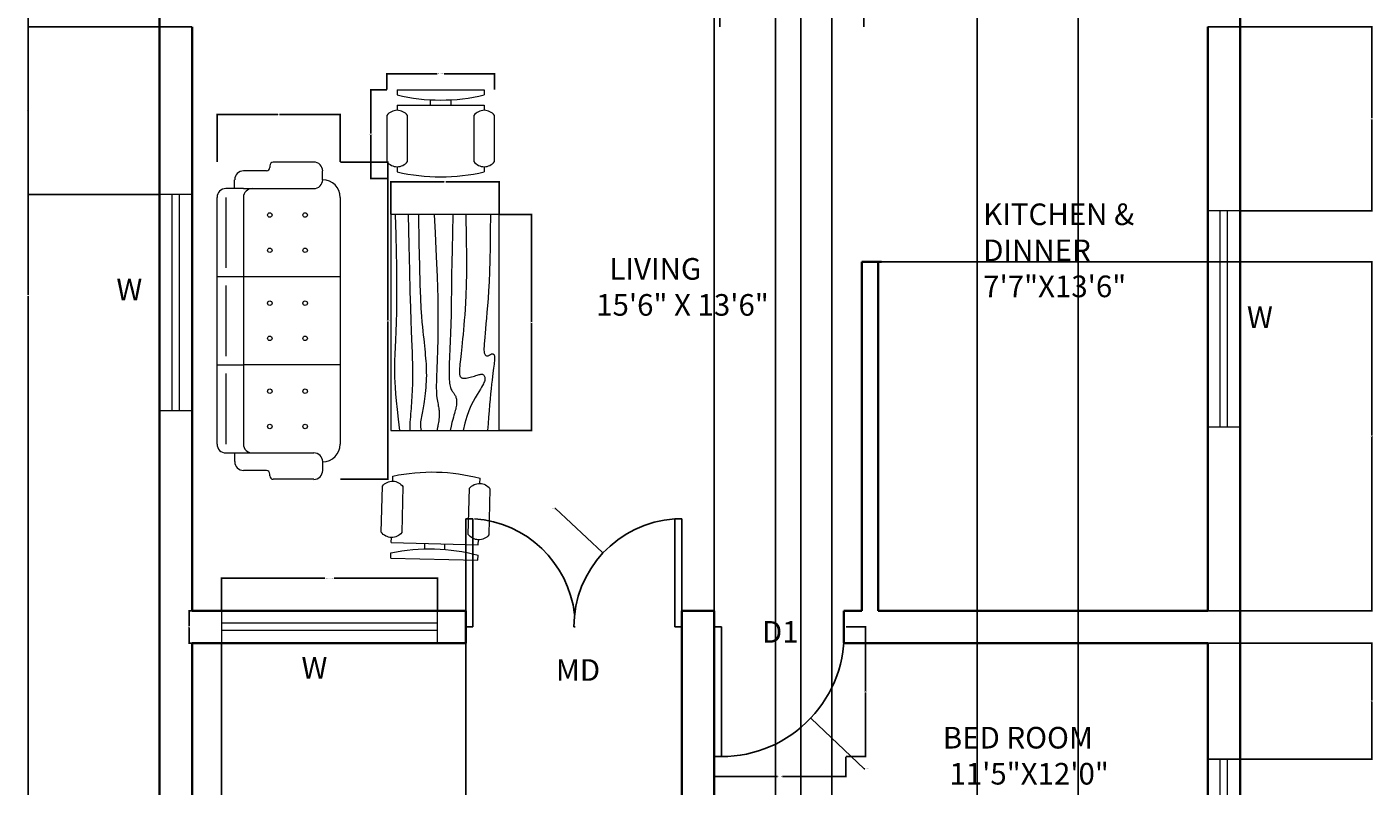
# Model space of a CAD drawing. Units: inches. Extents: x 2523 to 5630, y 2079 to 4208.
# Tile 2 of 3: x 2523 to 2897, y 2309 to 2520. Entities that reach past the tile are written whole.
import ezdxf

# ---------------------------------------------------------------- set-up
doc = ezdxf.new("R2010")
doc.units = ezdxf.units.IN
for name, color, linetype, lineweight in [('A-ANNO-DIMS', 2, 'Continuous', 18), ('A-ANNO-TEXT', 7, 'Continuous', 18), ('A-AREA-IDEN', 7, 'Continuous', 25), ('A-DOOR', 3, 'Continuous', 25), ('A-FURN', 8, 'Continuous', 18), ('A-GLAZ', 4, 'Continuous', 18), ('A-WALL', 7, 'Continuous', 35)]:
    doc.layers.add(name, color=color, linetype=linetype, lineweight=lineweight)
doc.styles.get("Standard").update_dxf_attribs({"font": 'arial.ttf'})
doc.dimstyles.get("Standard").update_dxf_attribs({"dimtxt": 0.18, "dimasz": 0.18, "dimexe": 0.18, "dimexo": 0.0625, "dimgap": 0.09, "dimtad": 0, "dimtih": 1, "dimtoh": 1, "dimdec": 4, "dimzin": 0, "dimdsep": 46, "dimtxsty": 'Standard', "dimcen": 0.09, "dimadec": 0, "dimazin": 0, "dimtfac": 1, "dimtdec": 4, "dimtofl": 0, "dimtmove": 0, "dimatfit": 3, "dimfxl": 1, "dimtolj": 1, "dimtzin": 0, "dimarcsym": 0})

# ---------------------------------------------------------------- blocks, each defined once
blk = doc.blocks.new('A$C1BE21B70')
for p, q in [((0.269, 0.942), (2.154, 0.942)), ((0.875, 0.942), (0.875, 0.875)), ((1.548, 0), (1.548, 0.942)), ((0.202, 0.875), (0.202, 0.74)), ((0.808, 0.875), (0.269, 0.875)), ((0.875, 0.875), (0.875, 0.74)), ((1.481, 0.875), (0.942, 0.875)), ((2.154, 0.875), (1.616, 0.875)), ((2.221, 0.74), (2.221, 0.875)), ((0.067, 0.565), (0.067, 0.74)), ((0.202, 0.808), (0.135, 0.808)), ((0.202, 0.74), (0.202, 0.202)), ((2.154, 0.74), (0.269, 0.74)), ((0.875, 0), (0.875, 0.74)), ((2.221, 0.808), (2.289, 0.808)), ((2.221, 0.74), (2.221, 0.202)), ((2.356, 0.565), (2.356, 0.74)), ((0.027, 0.539), (0.04, 0.539)), ((2.396, 0.539), (2.383, 0.539)), ((0, 0.202), (0, 0.512)), ((2.423, 0.202), (2.423, 0.512)), ((0.135, 0.135), (0.067, 0.135)), ((2.289, 0.135), (2.356, 0.135)), ((2.154, 0), (0.269, 0))]:
    blk.add_line(p, q)
for centre in [(0.404, 0.539), (0.673, 0.539), (1.077, 0.539), (1.346, 0.539), (1.75, 0.539), (2.019, 0.539), (0.404, 0.269), (0.673, 0.269), (1.077, 0.269), (1.346, 0.269), (1.75, 0.269), (2.019, 0.269)]:
    blk.add_circle(centre, 0.0171)
for centre, radius, start, end in [((0.269, 0.875), 0.0673, 90, 180), ((2.154, 0.875), 0.0673, 0, 90), ((0.135, 0.74), 0.0673, 90, 180), ((0.269, 0.673), 0.0673, 90, 180), ((2.154, 0.673), 0.0673, 0, 90), ((2.289, 0.74), 0.0673, 0, 90), ((0.027, 0.512), 0.0269, 90, 180), ((0.04, 0.565), 0.0269, 270, 0), ((2.383, 0.565), 0.0269, 180, 270), ((2.396, 0.512), 0.0269, 0, 90), ((0.067, 0.202), 0.0673, 180, 270), ((0.135, 0.202), 0.0673, 270, 0), ((0.269, 0.135), 0.135, 180, 270), ((2.154, 0.135), 0.135, 270, 0), ((2.289, 0.202), 0.0673, 180, 270), ((2.356, 0.202), 0.0673, 270, 0)]:
    blk.add_arc(centre, radius, start, end)
blk = doc.blocks.new('Table - Rectangular Woodgrain 60 x 30 in.')
for p, q in [((0, 0), (0, -30)), ((60, 0), (0, 0)), ((60, -30), (60, 0)), ((0, -30), (60, -30))]:
    blk.add_line(p, q)
for points in [[(0, -2.4), (4.8155, -2.418), (9.0302, -2.4688), (12.709, -2.5477), (15.9167, -2.65), (18.7181, -2.7711), (21.1781, -2.9063), (23.3616, -3.0508), (25.3333, -3.2), (27.1477, -3.3495), (28.8172, -3.4958), (30.3437, -3.636), (31.7291, -3.7667), (32.9756, -3.8849), (34.0849, -3.9875), (35.059, -4.0714), (35.9, -4.1334), (36.6114, -4.1711), (37.2041, -4.1854), (37.6906, -4.1779), (38.0833, -4.15), (38.3948, -4.1034), (38.6375, -4.0396), (38.8239, -3.9602), (38.9666, -3.8667), (39.0764, -3.7608), (39.1573, -3.6448), (39.2116, -3.521), (39.2416, -3.3917), (39.2498, -3.2593), (39.2385, -3.1261), (39.21, -2.9944), (39.1666, -2.8667), (39.111, -2.7447), (39.0468, -2.6281), (38.978, -2.5163), (38.9083, -2.4083), (38.8418, -2.3035), (38.7823, -2.201), (38.7337, -2.1001), (38.7, -2), (38.6844, -1.9003), (38.6875, -1.8021), (38.7094, -1.707), (38.75, -1.6167), (38.8094, -1.5326), (38.8875, -1.4563), (38.9844, -1.3893), (39.1, -1.3333), (39.2351, -1.2896), (39.3937, -1.2583), (39.5804, -1.2396), (39.8, -1.2333), (40.057, -1.2396), (40.3562, -1.2583), (40.7023, -1.2896), (41.1, -1.3333), (41.5547, -1.3895), (42.0755, -1.4573), (42.6721, -1.5361), (43.3542, -1.625), (44.1316, -1.7233), (45.014, -1.8302), (46.0114, -1.9449), (47.1333, -2.0667), (48.3862, -2.1947), (49.7625, -2.3281), (51.2513, -2.4663), (52.8416, -2.6083), (54.5226, -2.7535), (56.2833, -2.9011), (58.1127, -3.0501), (60, -3.2)], [(0, -9.2), (6.5759, -9.0858), (11.9385, -9.0365), (16.2527, -9.0418), (19.6833, -9.0917), (22.3952, -9.1759), (24.5531, -9.2844), (26.322, -9.4069), (27.8666, -9.5333), (29.3241, -9.6553), (30.7203, -9.7719), (32.0532, -9.8837), (33.3208, -9.9917), (34.5213, -10.0965), (35.6526, -10.199), (36.7128, -10.2999), (37.7, -10.4), (38.6129, -10.4996), (39.4531, -10.5969), (40.223, -10.6895), (40.925, -10.775), (41.5613, -10.8512), (42.1344, -10.9156), (42.6465, -10.966), (43.1, -11), (43.4976, -11.0158), (43.8437, -11.0136), (44.143, -10.9942), (44.4, -10.9583), (44.6195, -10.9069), (44.8062, -10.8406), (44.9648, -10.7603), (45.1, -10.6667), (45.2155, -10.5598), (45.3114, -10.4365), (45.3871, -10.2929), (45.4416, -10.125), (45.4743, -9.929), (45.4844, -9.7011), (45.4709, -9.4371), (45.4333, -9.1333), (45.3716, -8.7883), (45.2896, -8.4104), (45.1919, -8.0107), (45.0833, -7.6), (44.9685, -7.1893), (44.8521, -6.7896), (44.7388, -6.4117), (44.6333, -6.0667), (44.54, -5.7628), (44.4614, -5.4979), (44.4001, -5.2675), (44.3583, -5.0667), (44.3384, -4.8909), (44.3427, -4.7354), (44.3736, -4.5956), (44.4333, -4.4667), (44.5236, -4.3453), (44.6427, -4.2333), (44.7884, -4.1339), (44.9583, -4.05), (45.1501, -3.9849), (45.3614, -3.9417), (45.59, -3.9234), (45.8333, -3.9333), (46.0915, -3.9749), (46.3734, -4.0531), (46.6906, -4.1736), (47.0542, -4.3417), (47.4756, -4.5629), (47.9661, -4.8427), (48.5372, -5.1866), (49.2, -5.6), (49.9676, -6.0844), (50.8594, -6.625), (51.8965, -7.2031), (53.1, -7.8), (54.491, -8.3969), (56.0906, -8.975), (57.9199, -9.5156), (60, -10)], [(0, -12.8), (5.1847, -12.9322), (9.6213, -13.0323), (13.3963, -13.1059), (16.5958, -13.1583), (19.3063, -13.1952), (21.614, -13.2219), (23.6054, -13.2439), (25.3666, -13.2667), (26.9728, -13.2947), (28.4531, -13.3281), (29.8256, -13.3663), (31.1083, -13.4083), (32.3191, -13.4535), (33.476, -13.501), (34.597, -13.5501), (35.7, -13.6), (36.7984, -13.6497), (37.8875, -13.6979), (38.9578, -13.743), (40, -13.7833), (41.0047, -13.8174), (41.9625, -13.8438), (42.864, -13.8607), (43.7, -13.8667), (44.4631, -13.8604), (45.1552, -13.8417), (45.7801, -13.8104), (46.3416, -13.7667), (46.8439, -13.7104), (47.2906, -13.6417), (47.6858, -13.5604), (48.0333, -13.4667), (48.3375, -13.3608), (48.6042, -13.2448), (48.8396, -13.121), (49.05, -12.9917), (49.2417, -12.8593), (49.4208, -12.7261), (49.5937, -12.5944), (49.7667, -12.4667), (49.9452, -12.3451), (50.1323, -12.2313), (50.3303, -12.1268), (50.5416, -12.0333), (50.7686, -11.9524), (51.0135, -11.8854), (51.2788, -11.8341), (51.5666, -11.8), (51.8785, -11.7843), (52.2116, -11.7865), (52.562, -11.8059), (52.926, -11.8417), (53.2998, -11.8931), (53.6795, -11.9594), (54.0614, -12.0397), (54.4416, -12.1333), (54.8223, -12.2401), (55.2293, -12.3625), (55.6942, -12.5037), (56.2489, -12.6667), (56.9251, -12.8547), (57.7545, -13.0708), (58.7689, -13.3182), (60, -13.6)], [(0, -18), (5.124, -17.7273), (9.6609, -17.5057), (13.6705, -17.3303), (17.2125, -17.1958), (20.3467, -17.0973), (23.1328, -17.0297), (25.6307, -16.9878), (27.9, -16.9667), (29.9928, -16.9617), (31.9302, -16.9703), (33.7254, -16.9907), (35.3917, -17.0208), (36.9423, -17.0588), (38.3906, -17.1026), (39.7499, -17.1503), (41.0333, -17.2), (42.2519, -17.2496), (43.4073, -17.2969), (44.4986, -17.3395), (45.525, -17.375), (46.4858, -17.4012), (47.3802, -17.4156), (48.2074, -17.416), (48.9667, -17.4), (49.6583, -17.3662), (50.2872, -17.3167), (50.8595, -17.2547), (51.3812, -17.1833), (51.8584, -17.1057), (52.2971, -17.025), (52.7034, -16.9443), (53.0833, -16.8667), (53.443, -16.7951), (53.789, -16.7313), (54.128, -16.6768), (54.4666, -16.6334), (54.8115, -16.6024), (55.1693, -16.5854), (55.5465, -16.5841), (55.95, -16.6), (56.3828, -16.6337), (56.8346, -16.6823), (57.2915, -16.7418), (57.7396, -16.8084), (58.165, -16.878), (58.5539, -16.9469), (58.8924, -17.0111), (59.1666, -17.0667), (59.3679, -17.1107), (59.5078, -17.1438), (59.6032, -17.1675), (59.6708, -17.1833), (59.7275, -17.193), (59.7901, -17.1979), (59.8753, -17.1998), (60, -17.2)], [(0, -22.4), (8.0098, -22.2501), (14.4094, -22.1011), (19.4168, -21.9535), (23.25, -21.8083), (26.1269, -21.6663), (28.2656, -21.5281), (29.884, -21.3947), (31.2, -21.2667), (32.3967, -21.1448), (33.5172, -21.0292), (34.5697, -20.9198), (35.5625, -20.8167), (36.5037, -20.7198), (37.4015, -20.6292), (38.2642, -20.5448), (39.1, -20.4667), (39.9164, -20.3951), (40.7187, -20.3313), (41.5117, -20.2768), (42.3, -20.2333), (43.0883, -20.2024), (43.8812, -20.1854), (44.6836, -20.1841), (45.5, -20.2), (46.3328, -20.234), (47.1747, -20.2844), (48.0163, -20.3488), (48.8479, -20.425), (49.66, -20.5106), (50.4429, -20.6031), (51.1872, -20.7004), (51.8833, -20.8), (52.5246, -20.8999), (53.1166, -20.9995), (53.6681, -21.0983), (54.1875, -21.1958), (54.6834, -21.2919), (55.1646, -21.3859), (55.6394, -21.4777), (56.1167, -21.5667), (56.6028, -21.6515), (57.0961, -21.7266), (57.5929, -21.7852), (58.0896, -21.8208), (58.5823, -21.8268), (59.0674, -21.7964), (59.5412, -21.723), (60, -21.6)], [(0, -25.2), (8.6355, -25.0504), (15.7026, -24.9031), (21.4049, -24.7606), (25.9458, -24.625), (29.529, -24.4988), (32.3578, -24.3844), (34.6359, -24.284), (36.5667, -24.2), (38.3213, -24.1341), (39.9417, -24.0854), (41.437, -24.0523), (42.8167, -24.0333), (44.0901, -24.0268), (45.2667, -24.0313), (46.3557, -24.0451), (47.3667, -24.0667), (48.309, -24.0947), (49.1928, -24.1287), (50.0284, -24.168), (50.826, -24.2125), (51.5959, -24.2617), (52.3483, -24.3151), (53.0935, -24.3725), (53.8417, -24.4334), (54.6009, -24.497), (55.3699, -24.561), (56.1454, -24.6226), (56.9239, -24.6792), (57.7021, -24.7279), (58.4764, -24.7662), (59.2435, -24.7911), (60, -24.8)], [(0, -28.8), (5.6867, -28.6681), (10.45, -28.5698), (14.407, -28.5012), (17.675, -28.4584), (20.3711, -28.4374), (22.6125, -28.4344), (24.5164, -28.4455), (26.2, -28.4667), (27.762, -28.4947), (29.2276, -28.5281), (30.6033, -28.5663), (31.8958, -28.6084), (33.1118, -28.6535), (34.2578, -28.7011), (35.3405, -28.7501), (36.3666, -28.8), (37.3443, -28.8497), (38.288, -28.8974), (39.2137, -28.9412), (40.1375, -28.9792), (41.0753, -29.0093), (42.0432, -29.0297), (43.0572, -29.0384), (44.1333, -29.0333), (45.2936, -29.0114), (46.5843, -28.9641), (48.0579, -28.8816), (49.7666, -28.7542), (51.7629, -28.5721), (54.0989, -28.3255), (56.8272, -28.0048), (60, -27.6)]]:
    blk.add_lwpolyline(points)
blk = doc.blocks.new('Chair - Desk')
for p, q in [((-8.5, 0), (-8.5, -1)), ((-8.5, 0), (8.5, 0)), ((8.5, 0), (8.5, -1)), ((-2, -3), (-2, -1.9355)), ((2, -1.9576), (2, -3)), ((-10.5, -5), (-10.5, -14)), ((-8.5, -3), (-8.5, -4)), ((-8.5, -3), (8.5, -3)), ((-6.5, -14), (-6.5, -5)), ((6.5, -5), (6.5, -14)), ((8.5, -3), (8.5, -4)), ((10.5, -14), (10.5, -5)), ((-8.5, -15), (-8.5, -16)), ((8.5, -15), (8.5, -16))]:
    blk.add_line(p, q)
for centre, radius, start, end in [((0, 34.625), 36.625, 256.5803, 283.4197), ((-8.5, -6.5), 2.5, 36.8699, 143.1301), ((8.5, -6.5), 2.5, 36.8699, 143.1301), ((-8.5, -12.5), 2.5, 216.8699, 323.1301), ((8.5, -12.5), 2.5, 216.8699, 323.1301), ((0, 19.625), 36.625, 256.5803, 283.4197)]:
    blk.add_arc(centre, radius, start, end)
blk = doc.blocks.new('WIN-W-60IN')
for p, q in [((60, 5.5), (0, 5.5)), ((60, 3.5), (0, 3.5))]:
    blk.add_line(p, q)
blk.add_lwpolyline([(0, 0), (60, 0), (60, 9), (0, 9)], close=True)
blk = doc.blocks.new('DOOR-D1-36IN')
for p, q in [((2, 36), (0, 36)), ((2, 0), (2, 36)), ((0, 0), (2, 0))]:
    blk.add_line(p, q)
blk.add_arc((2, 34.06), 34.06, 270, 3.2732)
blk = doc.blocks.new('*D14')
at = {"layer": 'A-ANNO-DIMS', "color": 0, "lineweight": -2, "transparency": 16777216}
for p, q in [((2576.87, 2357.9), (2576.87, 2367.01)), ((2577.05, 2366.83), (2605.6, 2366.83)), ((2636.69, 2366.83), (2608.14, 2366.83)), ((2636.87, 2357.9), (2636.87, 2367.01))]:
    blk.add_line(p, q, dxfattribs=at)
at = {"layer": 'A-ANNO-DIMS', "color": 0, "transparency": 16777216}
for points in [[(2577.05, 2366.86), (2577.05, 2366.8), (2576.87, 2366.83)], [(2636.69, 2366.86), (2636.69, 2366.8), (2636.87, 2366.83)]]:
    blk.add_solid(points, dxfattribs=at)
at = {"layer": 'Defpoints', "color": 0, "transparency": 16777216}
for p in [(2636.87, 2366.83), (2576.87, 2357.83), (2636.87, 2357.83)]:
    blk.add_point(p, dxfattribs=at)
at = {"layer": 'A-ANNO-DIMS', "color": 0, "transparency": 16777216, "insert": (2606.87, 2366.83), "char_height": 0.18, "attachment_point": 5}
blk.add_mtext('\\A1;WINDOW W 60 TYP.', dxfattribs=at)
blk = doc.blocks.new('*D15')
at = {"layer": 'A-ANNO-DIMS', "color": 0, "lineweight": -2, "transparency": 16777216}
for p, q in [((2576.8, 2357.83), (2567.69, 2357.83)), ((2567.87, 2357.65), (2567.87, 2353.52)), ((2567.87, 2349.01), (2567.87, 2353.15)), ((2576.8, 2348.83), (2567.69, 2348.83))]:
    blk.add_line(p, q, dxfattribs=at)
at = {"layer": 'A-ANNO-DIMS', "color": 0, "transparency": 16777216}
for points in [[(2567.84, 2357.65), (2567.9, 2357.65), (2567.87, 2357.83)], [(2567.84, 2349.01), (2567.9, 2349.01), (2567.87, 2348.83)]]:
    blk.add_solid(points, dxfattribs=at)
at = {"layer": 'Defpoints', "color": 0, "transparency": 16777216}
for p in [(2567.87, 2357.83), (2576.87, 2357.83), (2576.87, 2348.83)]:
    blk.add_point(p, dxfattribs=at)
at = {"layer": 'A-ANNO-DIMS', "color": 0, "transparency": 16777216, "insert": (2567.87, 2353.33), "char_height": 0.18, "attachment_point": 5}
blk.add_mtext('\\A1;9 TYP.', dxfattribs=at)
blk = doc.blocks.new('*D22')
at = {"layer": 'A-ANNO-DIMS', "color": 0, "lineweight": -2, "transparency": 16777216}
for p, q in [((2713.69, 2317.27), (2713.69, 2311.67)), ((2750.23, 2317.27), (2750.23, 2311.67)), ((2713.87, 2311.85), (2731.24, 2311.85)), ((2750.05, 2311.85), (2732.68, 2311.85))]:
    blk.add_line(p, q, dxfattribs=at)
at = {"layer": 'A-ANNO-DIMS', "color": 0, "transparency": 16777216}
for points in [[(2713.87, 2311.88), (2713.87, 2311.82), (2713.69, 2311.85)], [(2750.05, 2311.88), (2750.05, 2311.82), (2750.23, 2311.85)]]:
    blk.add_solid(points, dxfattribs=at)
at = {"layer": 'Defpoints', "color": 0, "transparency": 16777216}
for p in [(2713.69, 2317.33), (2750.23, 2317.33), (2750.23, 2311.85)]:
    blk.add_point(p, dxfattribs=at)
at = {"layer": 'A-ANNO-DIMS', "color": 0, "transparency": 16777216, "insert": (2731.96, 2311.85), "char_height": 0.18, "attachment_point": 5}
blk.add_mtext('\\A1;D1 37 TYP.', dxfattribs=at)
blk = doc.blocks.new('*D23')
at = {"layer": 'A-ANNO-DIMS', "color": 0, "lineweight": -2, "transparency": 16777216}
for p, q in [((2750.29, 2353.33), (2755.89, 2353.33)), ((2755.71, 2353.15), (2755.71, 2335.52)), ((2755.71, 2317.51), (2755.71, 2335.15)), ((2750.29, 2317.33), (2755.89, 2317.33))]:
    blk.add_line(p, q, dxfattribs=at)
at = {"layer": 'A-ANNO-DIMS', "color": 0, "transparency": 16777216}
for points in [[(2755.68, 2353.15), (2755.74, 2353.15), (2755.71, 2353.33)], [(2755.68, 2317.51), (2755.74, 2317.51), (2755.71, 2317.33)]]:
    blk.add_solid(points, dxfattribs=at)
at = {"layer": 'Defpoints', "color": 0, "transparency": 16777216}
for p in [(2750.23, 2353.33), (2755.71, 2353.33), (2750.23, 2317.33)]:
    blk.add_point(p, dxfattribs=at)
at = {"layer": 'A-ANNO-DIMS', "color": 0, "transparency": 16777216, "insert": (2755.71, 2335.33), "char_height": 0.18, "attachment_point": 5}
blk.add_mtext('\\A1;36 TYP.', dxfattribs=at)
blk = doc.blocks.new('*D26')
at = {"layer": 'A-ANNO-DIMS', "color": 0, "lineweight": -2, "transparency": 16777216}
for p, q in [((2622.79, 2502.44), (2622.79, 2507.04)), ((2622.97, 2506.86), (2636.77, 2506.86)), ((2652.47, 2506.86), (2638.68, 2506.86)), ((2652.65, 2502.44), (2652.65, 2507.04))]:
    blk.add_line(p, q, dxfattribs=at)
at = {"layer": 'A-ANNO-DIMS', "color": 0, "transparency": 16777216}
for points in [[(2622.97, 2506.89), (2622.97, 2506.83), (2622.79, 2506.86)], [(2652.47, 2506.89), (2652.47, 2506.83), (2652.65, 2506.86)]]:
    blk.add_solid(points, dxfattribs=at)
at = {"layer": 'Defpoints', "color": 0, "transparency": 16777216}
for p in [(2652.65, 2506.86), (2622.79, 2502.38), (2652.65, 2502.38)]:
    blk.add_point(p, dxfattribs=at)
at = {"layer": 'A-ANNO-DIMS', "color": 0, "transparency": 16777216, "insert": (2637.72, 2506.86), "char_height": 0.18, "attachment_point": 5}
blk.add_mtext('\\A1;CHAIR 30 TYP.', dxfattribs=at)
blk = doc.blocks.new('*D27')
at = {"layer": 'A-ANNO-DIMS', "color": 0, "lineweight": -2, "transparency": 16777216}
for p, q in [((2622.73, 2502.38), (2618.13, 2502.38)), ((2618.31, 2502.2), (2618.31, 2490.24)), ((2618.31, 2477.91), (2618.31, 2489.88)), ((2622.73, 2477.73), (2618.13, 2477.73))]:
    blk.add_line(p, q, dxfattribs=at)
at = {"layer": 'A-ANNO-DIMS', "color": 0, "transparency": 16777216}
for points in [[(2618.28, 2502.2), (2618.34, 2502.2), (2618.31, 2502.38)], [(2618.28, 2477.91), (2618.34, 2477.91), (2618.31, 2477.73)]]:
    blk.add_solid(points, dxfattribs=at)
at = {"layer": 'Defpoints', "color": 0, "transparency": 16777216}
for p in [(2618.31, 2502.38), (2622.79, 2502.38), (2622.79, 2477.73)]:
    blk.add_point(p, dxfattribs=at)
at = {"layer": 'A-ANNO-DIMS', "color": 0, "transparency": 16777216, "insert": (2618.31, 2490.06), "char_height": 0.18, "attachment_point": 5}
blk.add_mtext('\\A1;25 TYP.', dxfattribs=at)
blk = doc.blocks.new('*D28')
at = {"layer": 'A-ANNO-DIMS', "color": 0, "lineweight": -2, "transparency": 16777216}
for p, q in [((2609.91, 2482.31), (2623.23, 2482.31)), ((2623.05, 2482.13), (2623.05, 2438.48)), ((2623.05, 2394.47), (2623.05, 2438.12)), ((2609.91, 2394.29), (2623.23, 2394.29))]:
    blk.add_line(p, q, dxfattribs=at)
at = {"layer": 'A-ANNO-DIMS', "color": 0, "transparency": 16777216}
for points in [[(2623.02, 2482.13), (2623.08, 2482.13), (2623.05, 2482.31)], [(2623.02, 2394.47), (2623.08, 2394.47), (2623.05, 2394.29)]]:
    blk.add_solid(points, dxfattribs=at)
at = {"layer": 'Defpoints', "color": 0, "transparency": 16777216}
for p in [(2609.85, 2482.31), (2623.05, 2482.31), (2609.85, 2394.29)]:
    blk.add_point(p, dxfattribs=at)
at = {"layer": 'A-ANNO-DIMS', "color": 0, "transparency": 16777216, "insert": (2623.05, 2438.3), "char_height": 0.18, "attachment_point": 5}
blk.add_mtext('\\A1;SOFA 88', dxfattribs=at)
blk = doc.blocks.new('*D29')
at = {"layer": 'A-ANNO-DIMS', "color": 0, "lineweight": -2, "transparency": 16777216}
for p, q in [((2575.62, 2482.37), (2575.62, 2495.7)), ((2575.8, 2495.52), (2592.52, 2495.52)), ((2609.67, 2495.52), (2592.95, 2495.52)), ((2609.85, 2482.37), (2609.85, 2495.7))]:
    blk.add_line(p, q, dxfattribs=at)
at = {"layer": 'A-ANNO-DIMS', "color": 0, "transparency": 16777216}
for points in [[(2575.8, 2495.55), (2575.8, 2495.49), (2575.62, 2495.52)], [(2609.67, 2495.55), (2609.67, 2495.49), (2609.85, 2495.52)]]:
    blk.add_solid(points, dxfattribs=at)
at = {"layer": 'Defpoints', "color": 0, "transparency": 16777216}
for p in [(2575.62, 2495.52), (2575.62, 2482.31), (2609.85, 2482.31)]:
    blk.add_point(p, dxfattribs=at)
at = {"layer": 'A-ANNO-DIMS', "color": 0, "transparency": 16777216, "insert": (2592.74, 2495.52), "char_height": 0.18, "attachment_point": 5}
blk.add_mtext('\\A1;34', dxfattribs=at)
blk = doc.blocks.new('*D30')
at = {"layer": 'A-ANNO-DIMS', "color": 0, "lineweight": -2, "transparency": 16777216}
for p, q in [((2653.99, 2467.81), (2663.1, 2467.81)), ((2662.92, 2467.63), (2662.92, 2437.99)), ((2662.92, 2407.99), (2662.92, 2437.63)), ((2653.99, 2407.81), (2663.1, 2407.81))]:
    blk.add_line(p, q, dxfattribs=at)
at = {"layer": 'A-ANNO-DIMS', "color": 0, "transparency": 16777216}
for points in [[(2662.89, 2467.63), (2662.95, 2467.63), (2662.92, 2467.81)], [(2662.89, 2407.99), (2662.95, 2407.99), (2662.92, 2407.81)]]:
    blk.add_solid(points, dxfattribs=at)
at = {"layer": 'Defpoints', "color": 0, "transparency": 16777216}
for p in [(2653.92, 2467.81), (2653.92, 2407.81), (2662.92, 2407.81)]:
    blk.add_point(p, dxfattribs=at)
at = {"layer": 'A-ANNO-DIMS', "color": 0, "transparency": 16777216, "insert": (2662.92, 2437.81), "char_height": 0.18, "attachment_point": 5}
blk.add_mtext('\\A1;TABLE 60', dxfattribs=at)
blk = doc.blocks.new('*D31')
at = {"layer": 'A-ANNO-DIMS', "color": 0, "lineweight": -2, "transparency": 16777216}
for p, q in [((2623.92, 2467.87), (2623.92, 2476.99)), ((2624.1, 2476.81), (2638.71, 2476.81)), ((2653.74, 2476.81), (2639.14, 2476.81)), ((2653.92, 2467.87), (2653.92, 2476.99))]:
    blk.add_line(p, q, dxfattribs=at)
at = {"layer": 'A-ANNO-DIMS', "color": 0, "transparency": 16777216}
for points in [[(2624.1, 2476.84), (2624.1, 2476.78), (2623.92, 2476.81)], [(2653.74, 2476.84), (2653.74, 2476.78), (2653.92, 2476.81)]]:
    blk.add_solid(points, dxfattribs=at)
at = {"layer": 'Defpoints', "color": 0, "transparency": 16777216}
for p in [(2653.92, 2476.81), (2623.92, 2467.81), (2653.92, 2467.81)]:
    blk.add_point(p, dxfattribs=at)
at = {"layer": 'A-ANNO-DIMS', "color": 0, "transparency": 16777216, "insert": (2638.92, 2476.81), "char_height": 0.18, "attachment_point": 5}
blk.add_mtext('\\A1;30', dxfattribs=at)
blk = doc.blocks.new('*D33')
at = {"layer": 'A-ANNO-DIMS', "color": 0, "lineweight": -2, "transparency": 16777216}
for p, q in [((2559.63, 2775.33), (2522.96, 2775.33)), ((2523.14, 2775.15), (2523.14, 2445.52)), ((2523.14, 2115.51), (2523.14, 2445.15)), ((2559.63, 2115.33), (2522.96, 2115.33))]:
    blk.add_line(p, q, dxfattribs=at)
at = {"layer": 'A-ANNO-DIMS', "color": 0, "transparency": 16777216}
for points in [[(2523.11, 2775.15), (2523.17, 2775.15), (2523.14, 2775.33)], [(2523.11, 2115.51), (2523.17, 2115.51), (2523.14, 2115.33)]]:
    blk.add_solid(points, dxfattribs=at)
at = {"layer": 'Defpoints', "color": 0, "transparency": 16777216}
for p in [(2523.14, 2775.33), (2559.69, 2775.33), (2559.69, 2115.33)]:
    blk.add_point(p, dxfattribs=at)
at = {"layer": 'A-ANNO-DIMS', "color": 0, "transparency": 16777216, "insert": (2523.14, 2445.33), "char_height": 0.18, "attachment_point": 5}
blk.add_mtext('\\A1;660', dxfattribs=at)
blk = doc.blocks.new('*D36')
at = {"layer": 'A-ANNO-DIMS', "color": 0, "lineweight": -2, "transparency": 16777216}
for p, q in [((2704.69, 2353.27), (2704.69, 2078.6)), ((2644.69, 2348.77), (2644.69, 2078.6)), ((2644.87, 2078.78), (2674.47, 2078.78)), ((2704.51, 2078.78), (2674.91, 2078.78))]:
    blk.add_line(p, q, dxfattribs=at)
at = {"layer": 'A-ANNO-DIMS', "color": 0, "transparency": 16777216}
for points in [[(2644.87, 2078.81), (2644.87, 2078.75), (2644.69, 2078.78)], [(2704.51, 2078.81), (2704.51, 2078.75), (2704.69, 2078.78)]]:
    blk.add_solid(points, dxfattribs=at)
at = {"layer": 'Defpoints', "color": 0, "transparency": 16777216}
for p in [(2704.69, 2353.33), (2644.69, 2348.83), (2704.69, 2078.78)]:
    blk.add_point(p, dxfattribs=at)
at = {"layer": 'A-ANNO-DIMS', "color": 0, "transparency": 16777216, "insert": (2674.69, 2078.78), "char_height": 0.18, "attachment_point": 5}
blk.add_mtext('\\A1;60', dxfattribs=at)
blk = doc.blocks.new('*D40')
at = {"layer": 'A-ANNO-DIMS', "color": 0, "lineweight": -2, "transparency": 16777216}
for p, q in [((2786.69, 2195.9), (2786.69, 2812.06)), ((2786.87, 2811.88), (2800.47, 2811.88)), ((2814.51, 2811.88), (2800.91, 2811.88)), ((2814.69, 2195.9), (2814.69, 2812.06))]:
    blk.add_line(p, q, dxfattribs=at)
at = {"layer": 'A-ANNO-DIMS', "color": 0, "transparency": 16777216}
for points in [[(2786.87, 2811.91), (2786.87, 2811.85), (2786.69, 2811.88)], [(2814.51, 2811.91), (2814.51, 2811.85), (2814.69, 2811.88)]]:
    blk.add_solid(points, dxfattribs=at)
at = {"layer": 'Defpoints', "color": 0, "transparency": 16777216}
for p in [(2814.69, 2811.88), (2786.69, 2195.83), (2814.69, 2195.83)]:
    blk.add_point(p, dxfattribs=at)
at = {"layer": 'A-ANNO-DIMS', "color": 0, "transparency": 16777216, "insert": (2800.69, 2811.88), "char_height": 0.18, "attachment_point": 5}
blk.add_mtext('\\A1;28', dxfattribs=at)
blk = doc.blocks.new('*D41')
at = {"layer": 'A-ANNO-DIMS', "color": 0, "lineweight": -2, "transparency": 16777216}
for p, q in [((2730.69, 2160.15), (2730.69, 2812.06)), ((2730.87, 2811.88), (2734.04, 2811.88)), ((2737.51, 2811.88), (2734.34, 2811.88)), ((2737.69, 2160.15), (2737.69, 2812.06))]:
    blk.add_line(p, q, dxfattribs=at)
at = {"layer": 'A-ANNO-DIMS', "color": 0, "transparency": 16777216}
for points in [[(2730.87, 2811.91), (2730.87, 2811.85), (2730.69, 2811.88)], [(2737.51, 2811.91), (2737.51, 2811.85), (2737.69, 2811.88)]]:
    blk.add_solid(points, dxfattribs=at)
at = {"layer": 'Defpoints', "color": 0, "transparency": 16777216}
for p in [(2737.69, 2811.88), (2730.69, 2160.08), (2737.69, 2160.08)]:
    blk.add_point(p, dxfattribs=at)
at = {"layer": 'A-ANNO-DIMS', "color": 0, "transparency": 16777216, "insert": (2734.19, 2811.88), "char_height": 0.18, "attachment_point": 5}
blk.add_mtext('\\A1;7', dxfattribs=at)
blk = doc.blocks.new('*D43')
at = {"layer": 'A-ANNO-DIMS', "color": 0, "lineweight": -2, "transparency": 16777216}
for p, q in [((2850.76, 2519.83), (2896.42, 2519.83)), ((2896.24, 2519.65), (2896.24, 2494.51)), ((2896.24, 2469.01), (2896.24, 2494.15)), ((2859.76, 2468.83), (2896.42, 2468.83))]:
    blk.add_line(p, q, dxfattribs=at)
at = {"layer": 'A-ANNO-DIMS', "color": 0, "transparency": 16777216}
for points in [[(2896.21, 2519.65), (2896.27, 2519.65), (2896.24, 2519.83)], [(2896.21, 2469.01), (2896.27, 2469.01), (2896.24, 2468.83)]]:
    blk.add_solid(points, dxfattribs=at)
at = {"layer": 'Defpoints', "color": 0, "transparency": 16777216}
for p in [(2850.69, 2519.83), (2896.24, 2519.83), (2859.69, 2468.83)]:
    blk.add_point(p, dxfattribs=at)
at = {"layer": 'A-ANNO-DIMS', "color": 0, "transparency": 16777216, "insert": (2896.24, 2494.33), "char_height": 0.18, "attachment_point": 5}
blk.add_mtext('\\A1;51.01', dxfattribs=at)
blk = doc.blocks.new('*D44')
at = {"layer": 'A-ANNO-DIMS', "color": 0, "lineweight": -2, "transparency": 16777216}
for p, q in [((2850.76, 2348.83), (2896.42, 2348.83)), ((2896.24, 2348.65), (2896.24, 2332.89)), ((2896.24, 2316.77), (2896.24, 2332.53)), ((2850.76, 2316.59), (2896.42, 2316.59))]:
    blk.add_line(p, q, dxfattribs=at)
at = {"layer": 'A-ANNO-DIMS', "color": 0, "transparency": 16777216}
for points in [[(2896.21, 2348.65), (2896.27, 2348.65), (2896.24, 2348.83)], [(2896.21, 2316.77), (2896.27, 2316.77), (2896.24, 2316.59)]]:
    blk.add_solid(points, dxfattribs=at)
at = {"layer": 'Defpoints', "color": 0, "transparency": 16777216}
for p in [(2850.69, 2348.83), (2896.24, 2348.83), (2850.69, 2316.59)]:
    blk.add_point(p, dxfattribs=at)
at = {"layer": 'A-ANNO-DIMS', "color": 0, "transparency": 16777216, "insert": (2896.24, 2332.71), "char_height": 0.18, "attachment_point": 5}
blk.add_mtext('\\A1;32.246', dxfattribs=at)
blk = doc.blocks.new('*D46')
at = {"layer": 'A-ANNO-DIMS', "color": 0, "lineweight": -2, "transparency": 16777216}
for p, q in [((2568.63, 2519.83), (2522.96, 2519.83)), ((2523.14, 2519.65), (2523.14, 2496.78)), ((2523.14, 2473.55), (2523.14, 2496.42)), ((2559.63, 2473.37), (2522.96, 2473.37))]:
    blk.add_line(p, q, dxfattribs=at)
at = {"layer": 'A-ANNO-DIMS', "color": 0, "transparency": 16777216}
for points in [[(2523.11, 2519.65), (2523.17, 2519.65), (2523.14, 2519.83)], [(2523.11, 2473.55), (2523.17, 2473.55), (2523.14, 2473.37)]]:
    blk.add_solid(points, dxfattribs=at)
at = {"layer": 'Defpoints', "color": 0, "transparency": 16777216}
for p in [(2523.14, 2519.83), (2568.69, 2519.83), (2559.69, 2473.37)]:
    blk.add_point(p, dxfattribs=at)
at = {"layer": 'A-ANNO-DIMS', "color": 0, "transparency": 16777216, "insert": (2523.14, 2496.6), "char_height": 0.18, "attachment_point": 5}
blk.add_mtext('\\A1;46.47', dxfattribs=at)
blk = doc.blocks.new('*D47')
at = {"layer": 'A-ANNO-DIMS', "color": 0, "lineweight": -2, "transparency": 16777216}
for p, q in [((2568.69, 2348.77), (2568.69, 2078.6)), ((2576.87, 2348.77), (2576.87, 2078.6)), ((2568.87, 2078.78), (2572.39, 2078.78)), ((2576.69, 2078.78), (2573.17, 2078.78))]:
    blk.add_line(p, q, dxfattribs=at)
at = {"layer": 'A-ANNO-DIMS', "color": 0, "transparency": 16777216}
for points in [[(2568.87, 2078.81), (2568.87, 2078.75), (2568.69, 2078.78)], [(2576.69, 2078.81), (2576.69, 2078.75), (2576.87, 2078.78)]]:
    blk.add_solid(points, dxfattribs=at)
at = {"layer": 'Defpoints', "color": 0, "transparency": 16777216}
for p in [(2568.69, 2348.83), (2576.87, 2348.83), (2576.87, 2078.78)]:
    blk.add_point(p, dxfattribs=at)
at = {"layer": 'A-ANNO-DIMS', "color": 0, "transparency": 16777216, "insert": (2572.78, 2078.78), "char_height": 0.18, "attachment_point": 5}
blk.add_mtext('\\A1;8.174', dxfattribs=at)
blk = doc.blocks.new('*D48')
at = {"layer": 'A-ANNO-DIMS', "color": 0, "lineweight": -2, "transparency": 16777216}
for p, q in [((2760.23, 2454.68), (2896.42, 2454.68)), ((2896.24, 2454.5), (2896.24, 2406.44)), ((2896.24, 2358.01), (2896.24, 2406.08)), ((2759.26, 2357.83), (2896.42, 2357.83))]:
    blk.add_line(p, q, dxfattribs=at)
at = {"layer": 'A-ANNO-DIMS', "color": 0, "transparency": 16777216}
for points in [[(2896.21, 2454.5), (2896.27, 2454.5), (2896.24, 2454.68)], [(2896.21, 2358.01), (2896.27, 2358.01), (2896.24, 2357.83)]]:
    blk.add_solid(points, dxfattribs=at)
at = {"layer": 'Defpoints', "color": 0, "transparency": 16777216}
for p in [(2760.16, 2454.68), (2759.19, 2357.83), (2896.24, 2357.83)]:
    blk.add_point(p, dxfattribs=at)
at = {"layer": 'A-ANNO-DIMS', "color": 0, "transparency": 16777216, "insert": (2896.24, 2406.26), "char_height": 0.18, "attachment_point": 5}
blk.add_mtext('\\A1;96.85', dxfattribs=at)
blk = doc.blocks.new('*D49')
at = {"layer": 'A-ANNO-DIMS', "color": 0, "lineweight": -2, "transparency": 16777216}
for p, q in [((2713.69, 2204.9), (2713.69, 2812.06)), ((2713.87, 2811.88), (2729.54, 2811.88)), ((2746.14, 2811.88), (2730.47, 2811.88)), ((2746.32, 2204.9), (2746.32, 2812.06))]:
    blk.add_line(p, q, dxfattribs=at)
at = {"layer": 'A-ANNO-DIMS', "color": 0, "transparency": 16777216}
for points in [[(2713.87, 2811.91), (2713.87, 2811.85), (2713.69, 2811.88)], [(2746.14, 2811.91), (2746.14, 2811.85), (2746.32, 2811.88)]]:
    blk.add_solid(points, dxfattribs=at)
at = {"layer": 'Defpoints', "color": 0, "transparency": 16777216}
for p in [(2746.32, 2811.88), (2713.69, 2204.83), (2746.32, 2204.83)]:
    blk.add_point(p, dxfattribs=at)
at = {"layer": 'A-ANNO-DIMS', "color": 0, "transparency": 16777216, "insert": (2730.01, 2811.88), "char_height": 0.18, "attachment_point": 5}
blk.add_mtext('\\A1;32.625', dxfattribs=at)
blk = doc.blocks.new('*D51')
at = {"layer": 'A-ANNO-DIMS', "color": 0, "lineweight": -2, "transparency": 16777216}
for p, q in [((2715.19, 2519.9), (2715.19, 2812.06)), ((2715.37, 2811.88), (2734.97, 2811.88)), ((2755.01, 2811.88), (2735.42, 2811.88)), ((2755.19, 2519.9), (2755.19, 2812.06))]:
    blk.add_line(p, q, dxfattribs=at)
at = {"layer": 'A-ANNO-DIMS', "color": 0, "transparency": 16777216}
for points in [[(2715.37, 2811.91), (2715.37, 2811.85), (2715.19, 2811.88)], [(2755.01, 2811.91), (2755.01, 2811.85), (2755.19, 2811.88)]]:
    blk.add_solid(points, dxfattribs=at)
at = {"layer": 'Defpoints', "color": 0, "transparency": 16777216}
for p in [(2755.19, 2811.88), (2715.19, 2519.83), (2755.19, 2519.83)]:
    blk.add_point(p, dxfattribs=at)
at = {"layer": 'A-ANNO-DIMS', "color": 0, "transparency": 16777216, "insert": (2735.19, 2811.88), "char_height": 0.18, "attachment_point": 5}
blk.add_mtext('\\A1;40', dxfattribs=at)
blk = doc.blocks.new('*D53')
at = {"layer": 'A-ANNO-DIMS', "color": 0, "lineweight": -2, "transparency": 16777216}
for p, q in [((2669.41, 2386.16), (2669.59, 2386.16)), ((2669.59, 2386.16), (2682.65, 2373.98)), ((2704.67, 2353.33), (2704.85, 2353.33)), ((2704.76, 2353.24), (2704.76, 2353.42))]:
    blk.add_line(p, q, dxfattribs=at)
at = {"layer": 'A-ANNO-DIMS', "color": 0, "transparency": 16777216}
blk.add_solid([(2682.67, 2374), (2682.63, 2373.95), (2682.78, 2373.85)], dxfattribs=at)
at = {"layer": 'Defpoints', "color": 0, "transparency": 16777216}
for p in [(2682.78, 2373.85), (2704.76, 2353.33)]:
    blk.add_point(p, dxfattribs=at)
at = {"layer": 'A-ANNO-DIMS', "color": 0, "transparency": 16777216, "insert": (2668.74, 2386.16), "char_height": 0.18, "attachment_point": 5}
blk.add_mtext('\\A1;2X R30.07', dxfattribs=at)
blk = doc.blocks.new('*D54')
at = {"layer": 'A-ANNO-DIMS', "color": 0, "lineweight": -2, "transparency": 16777216}
for p, q in [((2715.6, 2351.39), (2715.78, 2351.39)), ((2715.69, 2351.3), (2715.69, 2351.48)), ((2755.31, 2313.98), (2740.58, 2327.88)), ((2755.49, 2313.98), (2755.31, 2313.98))]:
    blk.add_line(p, q, dxfattribs=at)
at = {"layer": 'A-ANNO-DIMS', "color": 0, "transparency": 16777216}
blk.add_solid([(2740.6, 2327.9), (2740.56, 2327.86), (2740.45, 2328.01)], dxfattribs=at)
at = {"layer": 'Defpoints', "color": 0, "transparency": 16777216}
for p in [(2715.69, 2351.39), (2740.45, 2328.01)]:
    blk.add_point(p, dxfattribs=at)
at = {"layer": 'A-ANNO-DIMS', "color": 0, "transparency": 16777216, "insert": (2756.23, 2313.98), "char_height": 0.18, "attachment_point": 5}
blk.add_mtext('\\A1;3X R34.056', dxfattribs=at)

msp = doc.modelspace()

# ---------------------------------------------------------------- linework, layer by layer
at = {"layer": 'A-DOOR'}
for p, q in [((2644.693, 2353.334), (2644.693, 2383.334)), ((2644.693, 2383.334), (2646.693, 2383.334)), ((2646.693, 2383.334), (2646.693, 2353.334)), ((2704.693, 2383.334), (2702.693, 2383.334)), ((2702.693, 2383.334), (2702.693, 2353.334)), ((2704.693, 2353.334), (2704.693, 2383.334)), ((2644.693, 2353.334), (2646.693, 2353.334)), ((2674.693, 2353.334), (2675.0911, 2353.334)), ((2702.693, 2353.334), (2704.693, 2353.334)), ((2713.693, 2353.334), (2713.693, 2317.334))]:
    msp.add_line(p, q, dxfattribs=at)
for centre, start, end in [((2645.0197, 2353.334), 6.595683, 86.050132), ((2704.7645, 2353.334), 93.949868, 180)]:
    msp.add_arc(centre, 30.0714, start, end, dxfattribs=at)
at = {"layer": 'A-WALL'}
for p, q in [((2568.693, 2519.834), (2568.693, 2357.834)), ((2850.693, 2357.834), (2850.693, 2519.834)), ((2754.693, 2454.6846), (2754.693, 2357.834)), ((2760.1627, 2454.6846), (2754.693, 2454.6846)), ((2759.193, 2454.6846), (2759.193, 2357.834)), ((2644.693, 2357.834), (2568.693, 2357.834)), ((2644.693, 2348.834), (2644.693, 2357.834)), ((2704.693, 2195.834), (2704.693, 2357.834)), ((2713.693, 2357.834), (2704.693, 2357.834)), ((2713.693, 2204.834), (2713.693, 2357.834)), ((2754.693, 2357.834), (2749.693, 2357.834)), ((2749.693, 2348.834), (2749.693, 2357.834)), ((2850.693, 2357.834), (2759.193, 2357.834)), ((2644.693, 2348.834), (2568.693, 2348.834)), ((2568.693, 2348.834), (2568.693, 2124.334)), ((2850.693, 2348.834), (2749.693, 2348.834)), ((2850.693, 2204.834), (2850.693, 2348.834))]:
    msp.add_line(p, q, dxfattribs=at)
msp.add_lwpolyline([(2652.693, 2115.334), (2859.693, 2115.334), (2859.693, 2775.334), (2559.693, 2775.334), (2559.693, 2115.334), (2568.693, 2115.334)], dxfattribs=at)

# ---------------------------------------------------------------- block references
at = {"layer": 'A-DOOR'}
msp.add_blockref('DOOR-D1-36IN', (2713.693, 2317.334), dxfattribs=at)
at = {"layer": 'A-FURN', "xscale": 1.421988445322252, "yscale": 1.421988445322252, "zscale": 1.421988445322252}
msp.add_blockref('Chair - Desk', (2637.7225, 2502.3816), dxfattribs=at)
at = {"layer": 'A-FURN'}
for name, p, xscale, yscale, zscale, rotation in [('A$C1BE21B70', (2609.851, 2394.2916), 36.32324795298224, 36.32324795298224, 36.32324795298224, 90), ('Chair - Desk', (2635.9678, 2372.1427), -1.421988445322252, 1.421988445322252, 1.421988445322252, 178.5061869284156)]:
    msp.add_blockref(name, p, dxfattribs=dict(at, xscale=xscale, yscale=yscale, zscale=zscale, rotation=rotation))
at = {"layer": 'A-FURN', "rotation": 270}
msp.add_blockref('Table - Rectangular Woodgrain 60 x 30 in.', (2653.9239, 2467.8119), dxfattribs=at)
at = {"layer": 'A-GLAZ'}
for p, rotation in [((2559.693, 2473.3671), 269.9999999999993), ((2850.693, 2468.8271), 270.0000000000014), ((2850.693, 2316.5883), 270.0000000000015)]:
    msp.add_blockref('WIN-W-60IN', p, dxfattribs=dict(at, rotation=rotation))
msp.add_blockref('WIN-W-60IN', (2576.867, 2348.834), dxfattribs=at)

# ---------------------------------------------------------------- texts
at = {"layer": 'A-ANNO-TEXT', "char_height": 6, "attachment_point": 1}
for s, insert in [('W', (2547.681, 2449.9721)), ('W', (2861.5997, 2442.285)), ('D1', (2726.9345, 2354.9601)), ('W', (2599.0708, 2344.9593)), ('MD', (2669.7133, 2344.3717))]:
    msp.add_mtext_dynamic_manual_height_columns(s, width=48.58232, gutter_width=12.5, heights=[0], dxfattribs=dict(at, insert=insert))
at = {"layer": 'A-AREA-IDEN', "char_height": 6, "attachment_point": 1}
for s, width, heights, insert in [('KITCHEN &      DINNER \\P7\'7"X13\'6"', 57.081551, [38.5225], (2788.3564, 2470.8397)), ('  LIVING \\P15\'6" X 13\'6"', 48.58232, [0], (2680.9001, 2455.6951)), ('BED ROOM\\P 11\'5"X12\'0"', 48.58232, [0], (2777.154, 2325.5898))]:
    msp.add_mtext_dynamic_manual_height_columns(s, width=width, gutter_width=12.5, heights=heights, dxfattribs=dict(at, insert=insert))

# ---------------------------------------------------------------- dimensions: what is measured, and where the dimension line sits
at = {"layer": 'A-ANNO-DIMS'}
for base, p1, p2, override, picture, middle in [((2746.3179, 2811.884), (2713.693, 2204.834), (2746.3179, 2204.834), {"dimdec": 3, "dimlfac": 1, "dimrnd": 0, "dimzin": 0, "dimdsep": 46, "dimlunit": 2}, '*D49', (2730.0055, 2811.884)), ((2755.193, 2811.884), (2715.193, 2519.834), (2755.193, 2519.834), {"dimdec": 0, "dimlfac": 1, "dimrnd": 0, "dimzin": 0, "dimdsep": 46, "dimlunit": 2}, '*D51', (2735.193, 2811.884)), ((2737.693, 2811.884), (2730.693, 2160.084), (2737.693, 2160.084), {"dimdec": 0, "dimlfac": 1, "dimrnd": 0, "dimzin": 0, "dimdsep": 46, "dimlunit": 2}, '*D41', (2734.193, 2811.884)), ((2814.693, 2811.884), (2786.693, 2195.834), (2814.693, 2195.834), {"dimdec": 0, "dimlfac": 1, "dimrnd": 0, "dimzin": 0, "dimdsep": 46, "dimlunit": 2}, '*D40', (2800.693, 2811.884)), ((2653.9239, 2476.8119), (2623.9239, 2467.8119), (2653.9239, 2467.8119), {"dimdec": 0, "dimlfac": 1, "dimrnd": 0, "dimzin": 0, "dimdsep": 46, "dimlunit": 2}, '*D31', (2638.9239, 2476.8119)), ((2704.693, 2078.784), (2644.693, 2348.834), (2704.693, 2353.334), {"dimdec": 0, "dimlfac": 1, "dimrnd": 0, "dimzin": 0, "dimdsep": 46, "dimlunit": 2}, '*D36', (2674.693, 2078.784)), ((2576.867, 2078.784), (2568.693, 2348.834), (2576.867, 2348.834), {"dimdec": 3, "dimlfac": 1, "dimrnd": 0, "dimzin": 0, "dimdsep": 46, "dimlunit": 2}, '*D47', (2572.78, 2078.784))]:
    dim = msp.add_linear_dim(base=base, p1=p1, p2=p2, dimstyle='Standard', override=override, dxfattribs=at)
    dim.commit()
    dim.dimension.update_dxf_attribs({"geometry": picture, "text_midpoint": middle})
for base, p1, p2, angle, override, picture, middle in [((2523.143, 2775.334), (2559.693, 2115.334), (2559.693, 2775.334), 90, {"dimdec": 0, "dimlfac": 1, "dimrnd": 0, "dimzin": 0, "dimdsep": 46, "dimlunit": 2}, '*D33', (2523.143, 2445.334)), ((2523.143, 2519.834), (2559.693, 2473.3671), (2568.693, 2519.834), 90, {"dimdec": 2, "dimlfac": 1, "dimrnd": 0, "dimzin": 0, "dimdsep": 46, "dimlunit": 2}, '*D46', (2523.143, 2496.6006)), ((2896.243, 2519.834), (2859.693, 2468.827), (2850.693, 2519.834), 90, {"dimdec": 2, "dimlfac": 1, "dimrnd": 0, "dimzin": 0, "dimdsep": 46, "dimlunit": 2}, '*D43', (2896.243, 2494.3305)), ((2575.6201, 2495.515), (2609.851, 2482.312), (2575.6201, 2482.312), 180, {"dimdec": 0, "dimlfac": 1, "dimrnd": 0, "dimzin": 0, "dimdsep": 46, "dimlunit": 2}, '*D29', (2592.7356, 2495.515)), ((2896.243, 2357.834), (2760.1627, 2454.6846), (2759.193, 2357.834), 90, {"dimdec": 2, "dimlfac": 1, "dimrnd": 0, "dimzin": 0, "dimdsep": 46, "dimlunit": 2}, '*D48', (2896.243, 2406.2593)), ((2896.243, 2348.834), (2850.693, 2316.5883), (2850.693, 2348.834), 90, {"dimdec": 3, "dimlfac": 1, "dimrnd": 0, "dimzin": 0, "dimdsep": 46, "dimlunit": 2}, '*D44', (2896.243, 2332.7112))]:
    dim = msp.add_linear_dim(base=base, p1=p1, p2=p2, angle=angle, dimstyle='Standard', override=override, dxfattribs=at)
    dim.commit()
    dim.dimension.update_dxf_attribs({"geometry": picture, "text_midpoint": middle})
for base, p1, p2, text, picture, middle in [((2652.6534, 2506.8609), (2622.7916, 2502.3816), (2652.6534, 2502.3816), 'CHAIR <> TYP.', '*D26', (2637.7225, 2506.8609)), ((2636.867, 2366.834), (2576.867, 2357.834), (2636.867, 2357.834), 'WINDOW W <> TYP.', '*D14', (2606.867, 2366.834)), ((2750.228, 2311.8538), (2713.693, 2317.334), (2750.228, 2317.334), 'D1 <> TYP.', '*D22', (2731.9605, 2311.8538))]:
    dim = msp.add_linear_dim(base=base, p1=p1, p2=p2, text=text, dimstyle='Standard', override={"dimdec": 0, "dimlfac": 1, "dimrnd": 0, "dimzin": 0, "dimdsep": 46, "dimlunit": 2}, dxfattribs=at)
    dim.commit()
    dim.dimension.update_dxf_attribs({"geometry": picture, "text_midpoint": middle})
for base, p1, p2, angle, text, picture, middle in [((2618.3124, 2502.3816), (2622.7916, 2477.7338), (2622.7916, 2502.3816), 90, '<> TYP.', '*D27', (2618.3124, 2490.0577)), ((2623.054, 2482.312), (2609.851, 2394.2916), (2609.851, 2482.312), 90, 'SOFA <>', '*D28', (2623.054, 2438.3018)), ((2662.9239, 2407.8119), (2653.9239, 2467.8119), (2653.9239, 2407.8119), 270, 'TABLE <>', '*D30', (2662.9239, 2437.8119)), ((2567.867, 2357.834), (2576.867, 2348.834), (2576.867, 2357.834), 90, '<> TYP.', '*D15', (2567.867, 2353.334)), ((2755.7083, 2353.334), (2750.228, 2317.334), (2750.228, 2353.334), 90, '<> TYP.', '*D23', (2755.7083, 2335.334))]:
    dim = msp.add_linear_dim(base=base, p1=p1, p2=p2, angle=angle, text=text, dimstyle='Standard', override={"dimdec": 0, "dimlfac": 1, "dimrnd": 0, "dimzin": 0, "dimdsep": 46, "dimlunit": 2}, dxfattribs=at)
    dim.commit()
    dim.dimension.update_dxf_attribs({"geometry": picture, "text_midpoint": middle})
for center, mpoint, text, override, picture, middle in [((2704.7645, 2353.334), (2682.7806, 2373.8524), '2X <>', {"dimdec": 2, "dimlfac": 1, "dimrnd": 0, "dimzin": 0, "dimdsep": 46, "dimlunit": 2}, '*D53', (2668.7356, 2386.1633)), ((2715.693, 2351.3896), (2740.4518, 2328.0062), '3X <>', {"dimdec": 3, "dimlfac": 1, "dimrnd": 0, "dimzin": 0, "dimdsep": 46, "dimlunit": 2}, '*D54', (2756.2301, 2313.9761))]:
    dim = msp.add_radius_dim(center=center, mpoint=mpoint, text=text, dimstyle='Standard', override=override, dxfattribs=at)
    dim.commit()
    dim.dimension.update_dxf_attribs({"geometry": picture, "text_midpoint": middle, "dimtype": 164})

doc.saveas('drawing.dxf')
